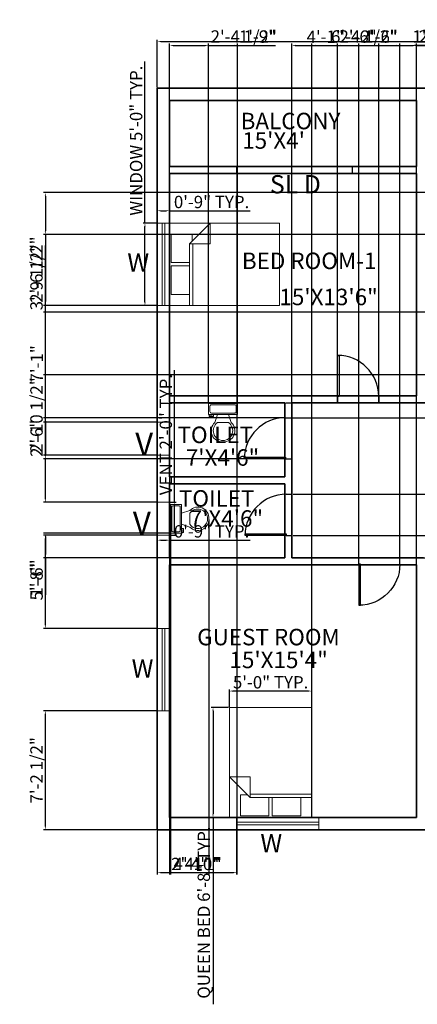
# Model space of a CAD drawing. Units: inches. Extents: x 3542 to 4275, y 1005 to 1722.
# Tile 1 of 6: x 3542 to 3831, y 1005 to 1722. Entities that reach past the tile are written whole.
import ezdxf

# ---------------------------------------------------------------- set-up
doc = ezdxf.new("R2010")
doc.units = ezdxf.units.IN
doc.layers.get('0').update_dxf_attribs({"color": 211})
for name, color, linetype, lineweight in [('A-ANNO-DIMS', 2, 'Continuous', 18), ('A-ANNO-TEXT', 7, 'Continuous', 18), ('A-AREA-IDEN', 7, 'Continuous', 25), ('A-DOOR', 3, 'Continuous', 25), ('A-FLOR-FIXT', 9, 'Continuous', 18), ('A-FURN', 8, 'Continuous', 18), ('A-GLAZ', 4, 'Continuous', 18), ('wall', 7, 'Continuous', 35)]:
    doc.layers.add(name, color=color, linetype=linetype, lineweight=lineweight)
doc.styles.get("Standard").update_dxf_attribs({"font": 'arial.ttf'})
doc.dimstyles.new('ISO-25', dxfattribs={"dimtxt": 9, "dimasz": 2.5, "dimexe": 1.25, "dimexo": 0.625, "dimtad": 1, "dimdec": 1, "dimlunit": 4, "dimtxsty": 'Standard', "dimcen": 2.5, "dimadec": 0, "dimazin": 0, "dimtfac": 1, "dimtdec": 1, "dimtmove": 0, "dimatfit": 3, "dimfxl": 1, "dimarcsym": 0})

# ---------------------------------------------------------------- blocks, each defined once
blk = doc.blocks.new('*U2')
for p, q in [((0, 0), (0, -6)), ((40, 0), (40, -6))]:
    blk.add_line(p, q)
blk.add_lwpolyline([(0, 0), (0, 40), (1.75, 40), (1.75, 0)], close=True)
blk.add_arc((0, 0), 40, 0, 90)
blk = doc.blocks.new('Bed - Queen')
for p, q in [((0, -80.00003), (0, 0)), ((0, 0), (59.99999, 0)), ((59.99999, 0), (59.99999, -80.00003)), ((7.99999, -1.2), (28.79998, -1.2)), ((7.99999, -14.4), (7.99999, -1.2)), ((28.79998, -1.2), (28.79998, -14.4)), ((31.19999, -1.2), (51.99999, -1.2)), ((31.19999, -14.4), (31.19999, -1.2)), ((51.99999, -1.2), (51.99999, -16.4)), ((0, -14.4), (44.8, -14.4)), ((44.8, -16.8), (0, -16.8)), ((59.99999, -29.6), (44.8, -14.4)), ((44.8, -14.4), (44.8, -29.6)), ((51.99999, -16.4), (46.79936, -16.4)), ((44.8, -29.6), (59.99999, -29.6)), ((59.99999, -80.00003), (0, -80.00003))]:
    blk.add_line(p, q)
blk = doc.blocks.new('*U11')
for p, q in [((9.5, -6), (9.5, -2)), ((-10, -8.5), (-8, -8.5)), ((-10, -9.5), (-10, -8.5)), ((-7, -9.5), (-10, -9.5)), ((-8, -8.5), (-8, -8)), ((-7, -8), (-7, -9.5)), ((-4, -8), (-6, -14)), ((4, -14), (-4, -14)), ((4, -8), (6, -14))]:
    blk.add_line(p, q)
blk.add_lwpolyline([(10.5, -8), (10.5, 0), (-10.5, 0), (-10.5, -8)], close=True)
for points in [[(-9.5, -2), (-9.5, -6)], [(8.5, -1), (-8.5, -1)], [(-8.5, -7), (8.5, -7)]]:
    blk.add_lwpolyline(points)
for centre, radius, start, end in [((-8.625, -1.875), 0.8839, 81.8699, 188.1301), ((-8.625, -6.125), 0.8839, 171.869898, 278.1301), ((8.625, -1.875), 0.8839, 351.8699, 98.1301), ((8.625, -6.125), 0.8839, 261.8699, 8.1301), ((-0.4772, -19.9188), 8.0953, 133.01722, 273.38), ((0.0374, -19.8731), 7.127, 124.50543, 269.7), ((-0.0373, -19.8731), 7.127, 270.3, 55.4946), ((0.4773, -19.9188), 8.0953, 266.62, 46.9828)]:
    blk.add_arc(centre, radius, start, end)
blk = doc.blocks.new('*D12')
at = {"layer": 'A-ANNO-DIMS', "color": 0, "lineweight": -2, "transparency": 16777216}
for p, q in [((3641.89, 1673.05), (3641.89, 1707.82)), ((4181.89, 1673.05), (4181.89, 1707.82)), ((3644.39, 1706.57), (4179.39, 1706.57))]:
    blk.add_line(p, q, dxfattribs=at)
at = {"layer": 'A-ANNO-DIMS', "color": 0, "transparency": 16777216}
for points in [[(3644.39, 1706.99), (3644.39, 1706.16), (3641.89, 1706.57)], [(4179.39, 1706.99), (4179.39, 1706.16), (4181.89, 1706.57)]]:
    blk.add_solid(points, dxfattribs=at)
at = {"layer": 'Defpoints', "color": 0, "transparency": 16777216}
for p in [(4181.89, 1706.57), (3641.89, 1672.43), (4181.89, 1672.43)]:
    blk.add_point(p, dxfattribs=at)
at = {"layer": 'A-ANNO-DIMS', "color": 0, "transparency": 16777216, "insert": (3911.89, 1711.77), "char_height": 9, "attachment_point": 5}
blk.add_mtext("45'", dxfattribs=at)
blk = doc.blocks.new('WIN-60IN')
for p, q in [((3.5, 60), (3.5, 0)), ((5.5, 60), (5.5, 0))]:
    blk.add_line(p, q)
blk.add_lwpolyline([(0, 60), (9, 60), (9, 0), (0, 0)], close=True)
blk = doc.blocks.new('DOOR-SLIDING-84IN')
blk.add_lwpolyline([(0, 0), (0, 5), (84, 5), (84, 0)], close=True)
blk = doc.blocks.new('VENT-24IN')
blk.add_lwpolyline([(0, 24), (9, 24), (9, 0), (0, 0)], close=True)
blk = doc.blocks.new('*D17')
at = {"layer": 'A-ANNO-DIMS', "color": 0, "lineweight": -2, "transparency": 16777216}
for p, q in [((3632.89, 1574.23), (3632.89, 1691.87)), ((3641.26, 1574.23), (3631.64, 1574.23)), ((3632.89, 1516.73), (3632.89, 1571.73)), ((3641.26, 1514.23), (3631.64, 1514.23))]:
    blk.add_line(p, q, dxfattribs=at)
at = {"layer": 'A-ANNO-DIMS', "color": 0, "transparency": 16777216}
for points in [[(3632.47, 1571.73), (3633.31, 1571.73), (3632.89, 1574.23)], [(3632.47, 1516.73), (3633.31, 1516.73), (3632.89, 1514.23)]]:
    blk.add_solid(points, dxfattribs=at)
at = {"layer": 'Defpoints', "color": 0, "transparency": 16777216}
for p in [(3632.89, 1574.23), (3641.89, 1574.23), (3641.89, 1514.23)]:
    blk.add_point(p, dxfattribs=at)
at = {"layer": 'A-ANNO-DIMS', "color": 0, "transparency": 16777216, "insert": (3627.61, 1634.3), "char_height": 9, "attachment_point": 5, "rotation": 90}
blk.add_mtext('WINDOW 5\'-0" TYP.', dxfattribs=at)
blk = doc.blocks.new('*D18')
at = {"layer": 'A-ANNO-DIMS', "color": 0, "lineweight": -2, "transparency": 16777216}
for p, q in [((3641.89, 1574.86), (3641.89, 1584.48)), ((3644.39, 1583.23), (3648.39, 1583.23)), ((3650.89, 1574.86), (3650.89, 1584.48)), ((3650.89, 1583.23), (3709.5, 1583.23))]:
    blk.add_line(p, q, dxfattribs=at)
at = {"layer": 'A-ANNO-DIMS', "color": 0, "transparency": 16777216}
for points in [[(3644.39, 1583.65), (3644.39, 1582.82), (3641.89, 1583.23)], [(3648.39, 1583.65), (3648.39, 1582.82), (3650.89, 1583.23)]]:
    blk.add_solid(points, dxfattribs=at)
at = {"layer": 'Defpoints', "color": 0, "transparency": 16777216}
for p in [(3650.89, 1583.23), (3641.89, 1574.23), (3650.89, 1574.23)]:
    blk.add_point(p, dxfattribs=at)
at = {"layer": 'A-ANNO-DIMS', "color": 0, "transparency": 16777216, "insert": (3681.44, 1588.45), "char_height": 9, "attachment_point": 5}
blk.add_mtext('0\'-9" TYP.', dxfattribs=at)
blk = doc.blocks.new('*D19')
at = {"layer": 'A-ANNO-DIMS', "color": 0, "lineweight": -2, "transparency": 16777216}
for p, q in [((3693.87, 1221.43), (3681.24, 1221.43)), ((3682.49, 1218.93), (3682.49, 1143.93)), ((3693.87, 1141.43), (3681.24, 1141.43)), ((3682.49, 1141.43), (3682.49, 1005.29))]:
    blk.add_line(p, q, dxfattribs=at)
at = {"layer": 'A-ANNO-DIMS', "color": 0, "transparency": 16777216}
for points in [[(3682.08, 1218.93), (3682.91, 1218.93), (3682.49, 1221.43)], [(3682.08, 1143.93), (3682.91, 1143.93), (3682.49, 1141.43)]]:
    blk.add_solid(points, dxfattribs=at)
at = {"layer": 'Defpoints', "color": 0, "transparency": 16777216}
for p in [(3694.49, 1221.43), (3682.49, 1141.43), (3694.49, 1141.43)]:
    blk.add_point(p, dxfattribs=at)
at = {"layer": 'A-ANNO-DIMS', "color": 0, "transparency": 16777216, "insert": (3676.94, 1072.11), "char_height": 9, "attachment_point": 5, "rotation": 90}
blk.add_mtext('QUEEN BED 6\'-8" TYP.', dxfattribs=at)
blk = doc.blocks.new('*D20')
at = {"layer": 'A-ANNO-DIMS', "color": 0, "lineweight": -2, "transparency": 16777216}
for p, q in [((3694.49, 1222.05), (3694.49, 1234.68)), ((3751.99, 1233.43), (3696.99, 1233.43)), ((3754.49, 1222.05), (3754.49, 1234.68))]:
    blk.add_line(p, q, dxfattribs=at)
at = {"layer": 'A-ANNO-DIMS', "color": 0, "transparency": 16777216}
for points in [[(3696.99, 1233.84), (3696.99, 1233.01), (3694.49, 1233.43)], [(3751.99, 1233.84), (3751.99, 1233.01), (3754.49, 1233.43)]]:
    blk.add_solid(points, dxfattribs=at)
at = {"layer": 'Defpoints', "color": 0, "transparency": 16777216}
for p in [(3694.49, 1233.43), (3694.49, 1221.43), (3754.49, 1221.43)]:
    blk.add_point(p, dxfattribs=at)
at = {"layer": 'A-ANNO-DIMS', "color": 0, "transparency": 16777216, "insert": (3724.49, 1238.65), "char_height": 9, "attachment_point": 5}
blk.add_mtext('5\'-0" TYP.', dxfattribs=at)
blk = doc.blocks.new('*D25')
at = {"layer": 'A-ANNO-DIMS', "color": 0, "lineweight": -2, "transparency": 16777216}
for p, q in [((3654.49, 1370.93), (3654.49, 1467.04)), ((3651.51, 1370.93), (3655.74, 1370.93)), ((3654.49, 1349.43), (3654.49, 1368.43)), ((3651.51, 1346.93), (3655.74, 1346.93))]:
    blk.add_line(p, q, dxfattribs=at)
at = {"layer": 'A-ANNO-DIMS', "color": 0, "transparency": 16777216}
for points in [[(3654.07, 1368.43), (3654.91, 1368.43), (3654.49, 1370.93)], [(3654.07, 1349.43), (3654.91, 1349.43), (3654.49, 1346.93)]]:
    blk.add_solid(points, dxfattribs=at)
at = {"layer": 'Defpoints', "color": 0, "transparency": 16777216}
for p in [(3650.89, 1370.93), (3654.49, 1370.93), (3650.89, 1346.93)]:
    blk.add_point(p, dxfattribs=at)
at = {"layer": 'A-ANNO-DIMS', "color": 0, "transparency": 16777216, "insert": (3649.27, 1420.23), "char_height": 9, "attachment_point": 5, "rotation": 90}
blk.add_mtext('VENT 2\'-0" TYP.', dxfattribs=at)
blk = doc.blocks.new('*D26')
at = {"layer": 'A-ANNO-DIMS', "color": 0, "lineweight": -2, "transparency": 16777216}
for p, q in [((3641.89, 1346.31), (3641.89, 1342.08)), ((3644.39, 1343.33), (3648.39, 1343.33)), ((3650.89, 1346.31), (3650.89, 1342.08)), ((3650.89, 1343.33), (3709.5, 1343.33))]:
    blk.add_line(p, q, dxfattribs=at)
at = {"layer": 'A-ANNO-DIMS', "color": 0, "transparency": 16777216}
for points in [[(3644.39, 1343.75), (3644.39, 1342.92), (3641.89, 1343.33)], [(3648.39, 1343.75), (3648.39, 1342.92), (3650.89, 1343.33)]]:
    blk.add_solid(points, dxfattribs=at)
at = {"layer": 'Defpoints', "color": 0, "transparency": 16777216}
for p in [(3641.89, 1346.93), (3650.89, 1346.93), (3650.89, 1343.33)]:
    blk.add_point(p, dxfattribs=at)
at = {"layer": 'A-ANNO-DIMS', "color": 0, "transparency": 16777216, "insert": (3681.44, 1348.55), "char_height": 9, "attachment_point": 5}
blk.add_mtext('0\'-9" TYP.', dxfattribs=at)
blk = doc.blocks.new('*D33')
at = {"layer": 'A-ANNO-DIMS', "color": 0, "lineweight": -2, "transparency": 16777216}
for p, q in [((3641.26, 1219.07), (3559.02, 1219.07)), ((3560.27, 1134.93), (3560.27, 1216.57)), ((3641.26, 1132.43), (3559.02, 1132.43))]:
    blk.add_line(p, q, dxfattribs=at)
at = {"layer": 'A-ANNO-DIMS', "color": 0, "transparency": 16777216}
for points in [[(3559.85, 1216.57), (3560.69, 1216.57), (3560.27, 1219.07)], [(3559.85, 1134.93), (3560.69, 1134.93), (3560.27, 1132.43)]]:
    blk.add_solid(points, dxfattribs=at)
at = {"layer": 'Defpoints', "color": 0, "transparency": 16777216}
for p in [(3560.27, 1219.07), (3641.89, 1219.07), (3641.89, 1132.43)]:
    blk.add_point(p, dxfattribs=at)
at = {"layer": 'A-ANNO-DIMS', "color": 0, "transparency": 16777216, "insert": (3554.99, 1175.75), "char_height": 9, "attachment_point": 5, "rotation": 90}
blk.add_mtext('7\'-2 1/2"', dxfattribs=at)
blk = doc.blocks.new('*D34')
at = {"layer": 'A-ANNO-DIMS', "color": 0, "lineweight": -2, "transparency": 16777216}
for p, q in [((3641.26, 1346.93), (3559.02, 1346.93)), ((3560.27, 1281.57), (3560.27, 1344.43)), ((3641.26, 1279.07), (3559.02, 1279.07))]:
    blk.add_line(p, q, dxfattribs=at)
at = {"layer": 'A-ANNO-DIMS', "color": 0, "transparency": 16777216}
for points in [[(3559.85, 1344.43), (3560.69, 1344.43), (3560.27, 1346.93)], [(3559.85, 1281.57), (3560.69, 1281.57), (3560.27, 1279.07)]]:
    blk.add_solid(points, dxfattribs=at)
at = {"layer": 'Defpoints', "color": 0, "transparency": 16777216}
for p in [(3560.27, 1346.93), (3641.89, 1346.93), (3641.89, 1279.07)]:
    blk.add_point(p, dxfattribs=at)
at = {"layer": 'A-ANNO-DIMS', "color": 0, "transparency": 16777216, "insert": (3555.05, 1313), "char_height": 9, "attachment_point": 5, "rotation": 90}
blk.add_mtext('5\'-8"', dxfattribs=at)
blk = doc.blocks.new('*D35')
at = {"layer": 'A-ANNO-DIMS', "color": 0, "lineweight": -2, "transparency": 16777216}
for p, q in [((3560.27, 1405.26), (3560.27, 1461.05)), ((3641.26, 1405.26), (3559.02, 1405.26)), ((3560.27, 1373.43), (3560.27, 1402.76)), ((3641.26, 1370.93), (3559.02, 1370.93))]:
    blk.add_line(p, q, dxfattribs=at)
at = {"layer": 'A-ANNO-DIMS', "color": 0, "transparency": 16777216}
for points in [[(3559.85, 1402.76), (3560.69, 1402.76), (3560.27, 1405.26)], [(3559.85, 1373.43), (3560.69, 1373.43), (3560.27, 1370.93)]]:
    blk.add_solid(points, dxfattribs=at)
at = {"layer": 'Defpoints', "color": 0, "transparency": 16777216}
for p in [(3560.27, 1405.26), (3641.89, 1405.26), (3641.89, 1370.93)]:
    blk.add_point(p, dxfattribs=at)
at = {"layer": 'A-ANNO-DIMS', "color": 0, "transparency": 16777216, "insert": (3554.99, 1434.41), "char_height": 9, "attachment_point": 5, "rotation": 90}
blk.add_mtext('2\'-10 1/2"', dxfattribs=at)
blk = doc.blocks.new('*D36')
at = {"layer": 'A-ANNO-DIMS', "color": 0, "lineweight": -2, "transparency": 16777216}
for p, q in [((3641.26, 1514.23), (3559.02, 1514.23)), ((3560.27, 1431.76), (3560.27, 1511.73)), ((3641.26, 1429.26), (3559.02, 1429.26))]:
    blk.add_line(p, q, dxfattribs=at)
at = {"layer": 'A-ANNO-DIMS', "color": 0, "transparency": 16777216}
for points in [[(3559.85, 1511.73), (3560.69, 1511.73), (3560.27, 1514.23)], [(3559.85, 1431.76), (3560.69, 1431.76), (3560.27, 1429.26)]]:
    blk.add_solid(points, dxfattribs=at)
at = {"layer": 'Defpoints', "color": 0, "transparency": 16777216}
for p in [(3560.27, 1514.23), (3641.89, 1514.23), (3641.89, 1429.26)]:
    blk.add_point(p, dxfattribs=at)
at = {"layer": 'A-ANNO-DIMS', "color": 0, "transparency": 16777216, "insert": (3555.13, 1471.75), "char_height": 9, "attachment_point": 5, "rotation": 90}
blk.add_mtext('7\'-1"', dxfattribs=at)
blk = doc.blocks.new('*D37')
at = {"layer": 'A-ANNO-DIMS', "color": 0, "lineweight": -2, "transparency": 16777216}
for p, q in [((3641.89, 1131.8), (3641.89, 1099.93)), ((3699.65, 1131.8), (3699.65, 1099.93)), ((3644.39, 1101.18), (3697.15, 1101.18))]:
    blk.add_line(p, q, dxfattribs=at)
at = {"layer": 'A-ANNO-DIMS', "color": 0, "transparency": 16777216}
for points in [[(3644.39, 1101.59), (3644.39, 1100.76), (3641.89, 1101.18)], [(3697.15, 1101.59), (3697.15, 1100.76), (3699.65, 1101.18)]]:
    blk.add_solid(points, dxfattribs=at)
at = {"layer": 'Defpoints', "color": 0, "transparency": 16777216}
for p in [(3641.89, 1132.43), (3699.65, 1132.43), (3699.65, 1101.18)]:
    blk.add_point(p, dxfattribs=at)
at = {"layer": 'A-ANNO-DIMS', "color": 0, "transparency": 16777216, "insert": (3670.77, 1106.4), "char_height": 9, "attachment_point": 5}
blk.add_mtext('4\'-10"', dxfattribs=at)
blk = doc.blocks.new('*D42')
at = {"layer": 'A-ANNO-DIMS', "color": 0, "lineweight": -2, "transparency": 16777216}
for p, q in [((3650.89, 1609.8), (3650.89, 1099.93)), ((3699.86, 1609.8), (3699.86, 1099.93)), ((3653.39, 1101.18), (3697.36, 1101.18))]:
    blk.add_line(p, q, dxfattribs=at)
at = {"layer": 'A-ANNO-DIMS', "color": 0, "transparency": 16777216}
for points in [[(3653.39, 1101.59), (3653.39, 1100.76), (3650.89, 1101.18)], [(3697.36, 1101.59), (3697.36, 1100.76), (3699.86, 1101.18)]]:
    blk.add_solid(points, dxfattribs=at)
at = {"layer": 'Defpoints', "color": 0, "transparency": 16777216}
for p in [(3650.89, 1610.43), (3699.86, 1610.43), (3699.86, 1101.18)]:
    blk.add_point(p, dxfattribs=at)
at = {"layer": 'A-ANNO-DIMS', "color": 0, "transparency": 16777216, "insert": (3675.37, 1106.32), "char_height": 9, "attachment_point": 5}
blk.add_mtext('4\'-1"', dxfattribs=at)
blk = doc.blocks.new('*D45')
at = {"layer": 'A-ANNO-DIMS', "color": 0, "lineweight": -2, "transparency": 16777216}
for p, q in [((3773.24, 1444.05), (3773.24, 1704.93)), ((3775.74, 1703.68), (3800.74, 1703.68)), ((3803.24, 1444.05), (3803.24, 1704.93))]:
    blk.add_line(p, q, dxfattribs=at)
at = {"layer": 'A-ANNO-DIMS', "color": 0, "transparency": 16777216}
for points in [[(3775.74, 1704.09), (3775.74, 1703.26), (3773.24, 1703.68)], [(3800.74, 1704.09), (3800.74, 1703.26), (3803.24, 1703.68)]]:
    blk.add_solid(points, dxfattribs=at)
at = {"layer": 'Defpoints', "color": 0, "transparency": 16777216}
for p in [(3803.24, 1703.68), (3773.24, 1443.43), (3803.24, 1443.43)]:
    blk.add_point(p, dxfattribs=at)
at = {"layer": 'A-ANNO-DIMS', "color": 0, "transparency": 16777216, "insert": (3788.24, 1708.9), "char_height": 9, "attachment_point": 5}
blk.add_mtext('2\'-6"', dxfattribs=at)
blk = doc.blocks.new('*D46')
at = {"layer": 'A-ANNO-DIMS', "color": 0, "lineweight": -2, "transparency": 16777216}
for p, q in [((3803.24, 1444.05), (3803.24, 1704.93)), ((3805.74, 1703.68), (3828.39, 1703.68)), ((3830.89, 1449.05), (3830.89, 1704.93)), ((3830.89, 1703.68), (3879.69, 1703.68))]:
    blk.add_line(p, q, dxfattribs=at)
at = {"layer": 'A-ANNO-DIMS', "color": 0, "transparency": 16777216}
for points in [[(3805.74, 1704.09), (3805.74, 1703.26), (3803.24, 1703.68)], [(3828.39, 1704.09), (3828.39, 1703.26), (3830.89, 1703.68)]]:
    blk.add_solid(points, dxfattribs=at)
at = {"layer": 'Defpoints', "color": 0, "transparency": 16777216}
for p in [(3830.89, 1703.68), (3803.24, 1443.43), (3830.89, 1448.43)]:
    blk.add_point(p, dxfattribs=at)
at = {"layer": 'A-ANNO-DIMS', "color": 0, "transparency": 16777216, "insert": (3856.54, 1708.96), "char_height": 9, "attachment_point": 5}
blk.add_mtext('2\'-3 1/2"', dxfattribs=at)
blk = doc.blocks.new('*D54')
at = {"layer": 'A-ANNO-DIMS', "color": 0, "lineweight": -2, "transparency": 16777216}
for p, q in [((4047.2, 1596.46), (3559.02, 1596.46)), ((3560.27, 1593.96), (3560.27, 1568.52)), ((4047.2, 1566.02), (3559.02, 1566.02)), ((3560.27, 1566.02), (3560.27, 1517.22))]:
    blk.add_line(p, q, dxfattribs=at)
at = {"layer": 'A-ANNO-DIMS', "color": 0, "transparency": 16777216}
for points in [[(3559.85, 1593.96), (3560.69, 1593.96), (3560.27, 1596.46)], [(3559.85, 1568.52), (3560.69, 1568.52), (3560.27, 1566.02)]]:
    blk.add_solid(points, dxfattribs=at)
at = {"layer": 'Defpoints', "color": 0, "transparency": 16777216}
for p in [(4047.82, 1596.46), (3560.27, 1566.02), (4047.82, 1566.02)]:
    blk.add_point(p, dxfattribs=at)
at = {"layer": 'A-ANNO-DIMS', "color": 0, "transparency": 16777216, "insert": (3554.99, 1540.37), "char_height": 9, "attachment_point": 5, "rotation": 90}
blk.add_mtext('2\'-6 1/2"', dxfattribs=at)
blk = doc.blocks.new('*D55')
at = {"layer": 'A-ANNO-DIMS', "color": 0, "lineweight": -2, "transparency": 16777216}
for p, q in [((3560.27, 1509.3), (3560.27, 1557.94)), ((4047.2, 1509.3), (3559.02, 1509.3)), ((3560.27, 1466.15), (3560.27, 1506.8)), ((4047.2, 1463.65), (3559.02, 1463.65))]:
    blk.add_line(p, q, dxfattribs=at)
at = {"layer": 'A-ANNO-DIMS', "color": 0, "transparency": 16777216}
for points in [[(3559.85, 1506.8), (3560.69, 1506.8), (3560.27, 1509.3)], [(3559.85, 1466.15), (3560.69, 1466.15), (3560.27, 1463.65)]]:
    blk.add_solid(points, dxfattribs=at)
at = {"layer": 'Defpoints', "color": 0, "transparency": 16777216}
for p in [(3560.27, 1509.3), (4047.82, 1509.3), (4047.82, 1463.65)]:
    blk.add_point(p, dxfattribs=at)
at = {"layer": 'A-ANNO-DIMS', "color": 0, "transparency": 16777216, "insert": (3554.99, 1534.87), "char_height": 9, "attachment_point": 5, "rotation": 90}
blk.add_mtext('3\'-9 1/2"', dxfattribs=at)
blk = doc.blocks.new('*D61')
at = {"layer": 'A-ANNO-DIMS', "color": 0, "lineweight": -2, "transparency": 16777216}
for p, q in [((3877.16, 1703.68), (3829.36, 1703.68)), ((3877.16, 1207.47), (3877.16, 1704.93)), ((3893.39, 1703.68), (3879.66, 1703.68)), ((3895.89, 1207.05), (3895.89, 1704.93))]:
    blk.add_line(p, q, dxfattribs=at)
at = {"layer": 'A-ANNO-DIMS', "color": 0, "transparency": 16777216}
for points in [[(3879.66, 1704.09), (3879.66, 1703.26), (3877.16, 1703.68)], [(3893.39, 1704.09), (3893.39, 1703.26), (3895.89, 1703.68)]]:
    blk.add_solid(points, dxfattribs=at)
at = {"layer": 'Defpoints', "color": 0, "transparency": 16777216}
for p in [(3877.16, 1703.68), (3877.16, 1206.85), (3895.89, 1206.43)]:
    blk.add_point(p, dxfattribs=at)
at = {"layer": 'A-ANNO-DIMS', "color": 0, "transparency": 16777216, "insert": (3852.01, 1708.96), "char_height": 9, "attachment_point": 5}
blk.add_mtext('1\'-6 1/2"', dxfattribs=at)
blk = doc.blocks.new('*D62')
at = {"layer": 'A-ANNO-DIMS', "color": 0, "lineweight": -2, "transparency": 16777216}
for p, q in [((3739.89, 1331.05), (3739.89, 1704.93)), ((3742.39, 1703.68), (3786.19, 1703.68)), ((3788.69, 1330.99), (3788.69, 1704.93))]:
    blk.add_line(p, q, dxfattribs=at)
at = {"layer": 'A-ANNO-DIMS', "color": 0, "transparency": 16777216}
for points in [[(3742.39, 1704.09), (3742.39, 1703.26), (3739.89, 1703.68)], [(3786.19, 1704.09), (3786.19, 1703.26), (3788.69, 1703.68)]]:
    blk.add_solid(points, dxfattribs=at)
at = {"layer": 'Defpoints', "color": 0, "transparency": 16777216}
for p in [(3788.69, 1703.68), (3739.89, 1330.43), (3788.69, 1330.37)]:
    blk.add_point(p, dxfattribs=at)
at = {"layer": 'A-ANNO-DIMS', "color": 0, "transparency": 16777216, "insert": (3764.29, 1708.82), "char_height": 9, "attachment_point": 5}
blk.add_mtext('4\'-1"', dxfattribs=at)
blk = doc.blocks.new('*D63')
at = {"layer": 'A-ANNO-DIMS', "color": 0, "lineweight": -2, "transparency": 16777216}
for p, q in [((3788.69, 1330.99), (3788.69, 1704.93)), ((3791.19, 1703.68), (3816.19, 1703.68)), ((3818.69, 1330.99), (3818.69, 1704.93))]:
    blk.add_line(p, q, dxfattribs=at)
at = {"layer": 'A-ANNO-DIMS', "color": 0, "transparency": 16777216}
for points in [[(3791.19, 1704.09), (3791.19, 1703.26), (3788.69, 1703.68)], [(3816.19, 1704.09), (3816.19, 1703.26), (3818.69, 1703.68)]]:
    blk.add_solid(points, dxfattribs=at)
at = {"layer": 'Defpoints', "color": 0, "transparency": 16777216}
for p in [(3818.69, 1703.68), (3788.69, 1330.37), (3818.69, 1330.37)]:
    blk.add_point(p, dxfattribs=at)
at = {"layer": 'A-ANNO-DIMS', "color": 0, "transparency": 16777216, "insert": (3803.69, 1708.9), "char_height": 9, "attachment_point": 5}
blk.add_mtext('2\'-6"', dxfattribs=at)
blk = doc.blocks.new('*D64')
at = {"layer": 'A-ANNO-DIMS', "color": 0, "lineweight": -2, "transparency": 16777216}
for p, q in [((3741.01, 1376.72), (4214.39, 1376.72)), ((4213.14, 1374.22), (4213.14, 1349.22)), ((3741.01, 1346.72), (4214.39, 1346.72))]:
    blk.add_line(p, q, dxfattribs=at)
at = {"layer": 'A-ANNO-DIMS', "color": 0, "transparency": 16777216}
for points in [[(4212.72, 1374.22), (4213.56, 1374.22), (4213.14, 1376.72)], [(4212.72, 1349.22), (4213.56, 1349.22), (4213.14, 1346.72)]]:
    blk.add_solid(points, dxfattribs=at)
at = {"layer": 'Defpoints', "color": 0, "transparency": 16777216}
for p in [(3740.38, 1376.72), (3740.38, 1346.72), (4213.14, 1346.72)]:
    blk.add_point(p, dxfattribs=at)
at = {"layer": 'A-ANNO-DIMS', "color": 0, "transparency": 16777216, "insert": (4207.92, 1361.72), "char_height": 9, "attachment_point": 5, "rotation": 90}
blk.add_mtext('2\'-6"', dxfattribs=at)
blk = doc.blocks.new('*D65')
at = {"layer": 'A-ANNO-DIMS', "color": 0, "lineweight": -2, "transparency": 16777216}
for p, q in [((3734.7, 1432.53), (3559.02, 1432.53)), ((3560.27, 1430.03), (3560.27, 1405.03)), ((3734.7, 1402.53), (3559.02, 1402.53))]:
    blk.add_line(p, q, dxfattribs=at)
at = {"layer": 'A-ANNO-DIMS', "color": 0, "transparency": 16777216}
for points in [[(3559.85, 1430.03), (3560.69, 1430.03), (3560.27, 1432.53)], [(3559.85, 1405.03), (3560.69, 1405.03), (3560.27, 1402.53)]]:
    blk.add_solid(points, dxfattribs=at)
at = {"layer": 'Defpoints', "color": 0, "transparency": 16777216}
for p in [(3735.32, 1432.53), (3560.27, 1402.53), (3735.32, 1402.53)]:
    blk.add_point(p, dxfattribs=at)
at = {"layer": 'A-ANNO-DIMS', "color": 0, "transparency": 16777216, "insert": (3555.05, 1417.53), "char_height": 9, "attachment_point": 5, "rotation": 90}
blk.add_mtext('2\'-6"', dxfattribs=at)
blk = doc.blocks.new('*D66')
at = {"layer": 'A-ANNO-DIMS', "color": 0, "lineweight": -2, "transparency": 16777216}
for p, q in [((3735.51, 1443.43), (4214.39, 1443.43)), ((4213.14, 1440.93), (4213.14, 1435.03)), ((3735.95, 1432.53), (4214.39, 1432.53)), ((4213.14, 1432.53), (4213.14, 1397.86))]:
    blk.add_line(p, q, dxfattribs=at)
at = {"layer": 'A-ANNO-DIMS', "color": 0, "transparency": 16777216}
for points in [[(4212.72, 1440.93), (4213.56, 1440.93), (4213.14, 1443.43)], [(4212.72, 1435.03), (4213.56, 1435.03), (4213.14, 1432.53)]]:
    blk.add_solid(points, dxfattribs=at)
at = {"layer": 'Defpoints', "color": 0, "transparency": 16777216}
for p in [(3734.89, 1443.43), (3735.32, 1432.53), (4213.14, 1432.53)]:
    blk.add_point(p, dxfattribs=at)
at = {"layer": 'A-ANNO-DIMS', "color": 0, "transparency": 16777216, "insert": (4207.92, 1413.94), "char_height": 9, "attachment_point": 5, "rotation": 90}
blk.add_mtext('0\'-11"', dxfattribs=at)
blk = doc.blocks.new('*D67')
at = {"layer": 'A-ANNO-DIMS', "color": 0, "lineweight": -2, "transparency": 16777216}
for p, q in [((4213.14, 1346.72), (4213.14, 1394.52)), ((3741.01, 1346.72), (4214.39, 1346.72)), ((4213.14, 1332.93), (4213.14, 1344.22)), ((3740.51, 1330.43), (4214.39, 1330.43))]:
    blk.add_line(p, q, dxfattribs=at)
at = {"layer": 'A-ANNO-DIMS', "color": 0, "transparency": 16777216}
for points in [[(4212.72, 1344.22), (4213.56, 1344.22), (4213.14, 1346.72)], [(4212.72, 1332.93), (4213.56, 1332.93), (4213.14, 1330.43)]]:
    blk.add_solid(points, dxfattribs=at)
at = {"layer": 'Defpoints', "color": 0, "transparency": 16777216}
for p in [(3740.38, 1346.72), (4213.14, 1346.72), (3739.89, 1330.43)]:
    blk.add_point(p, dxfattribs=at)
at = {"layer": 'A-ANNO-DIMS', "color": 0, "transparency": 16777216, "insert": (4207.86, 1371.87), "char_height": 9, "attachment_point": 5, "rotation": 90}
blk.add_mtext('1\'-4 1/2"', dxfattribs=at)
blk = doc.blocks.new('*D68')
at = {"layer": 'A-ANNO-DIMS', "color": 0, "lineweight": -2, "transparency": 16777216}
for p, q in [((3679.29, 1443.55), (3679.29, 1704.93)), ((3681.79, 1703.68), (3697.79, 1703.68)), ((3700.29, 1443.55), (3700.29, 1704.93)), ((3700.29, 1703.68), (3727.12, 1703.68))]:
    blk.add_line(p, q, dxfattribs=at)
at = {"layer": 'A-ANNO-DIMS', "color": 0, "transparency": 16777216}
for points in [[(3681.79, 1704.09), (3681.79, 1703.26), (3679.29, 1703.68)], [(3697.79, 1704.09), (3697.79, 1703.26), (3700.29, 1703.68)]]:
    blk.add_solid(points, dxfattribs=at)
at = {"layer": 'Defpoints', "color": 0, "transparency": 16777216}
for p in [(3700.29, 1703.68), (3679.29, 1442.92), (3700.29, 1442.92)]:
    blk.add_point(p, dxfattribs=at)
at = {"layer": 'A-ANNO-DIMS', "color": 0, "transparency": 16777216, "insert": (3714.96, 1708.9), "char_height": 9, "attachment_point": 5}
blk.add_mtext('1\'-9"', dxfattribs=at)
blk = doc.blocks.new('*D69')
at = {"layer": 'A-ANNO-DIMS', "color": 0, "lineweight": -2, "transparency": 16777216}
for p, q in [((3650.89, 1444.05), (3650.89, 1704.93)), ((3653.39, 1703.68), (3676.79, 1703.68)), ((3679.29, 1443.55), (3679.29, 1704.93)), ((3679.29, 1703.68), (3728.09, 1703.68))]:
    blk.add_line(p, q, dxfattribs=at)
at = {"layer": 'A-ANNO-DIMS', "color": 0, "transparency": 16777216}
for points in [[(3653.39, 1704.09), (3653.39, 1703.26), (3650.89, 1703.68)], [(3676.79, 1704.09), (3676.79, 1703.26), (3679.29, 1703.68)]]:
    blk.add_solid(points, dxfattribs=at)
at = {"layer": 'Defpoints', "color": 0, "transparency": 16777216}
for p in [(3679.29, 1703.68), (3650.89, 1443.43), (3679.29, 1442.92)]:
    blk.add_point(p, dxfattribs=at)
at = {"layer": 'A-ANNO-DIMS', "color": 0, "transparency": 16777216, "insert": (3704.94, 1708.96), "char_height": 9, "attachment_point": 5}
blk.add_mtext('2\'-4 1/2"', dxfattribs=at)
blk = doc.blocks.new('*D70')
at = {"layer": 'A-ANNO-DIMS', "color": 0, "lineweight": -2, "transparency": 16777216}
for p, q in [((3651.52, 1368.77), (3651.52, 1099.93)), ((3679.52, 1358.27), (3679.52, 1099.93)), ((3654.02, 1101.18), (3677.02, 1101.18))]:
    blk.add_line(p, q, dxfattribs=at)
at = {"layer": 'A-ANNO-DIMS', "color": 0, "transparency": 16777216}
for points in [[(3654.02, 1101.59), (3654.02, 1100.76), (3651.52, 1101.18)], [(3677.02, 1101.59), (3677.02, 1100.76), (3679.52, 1101.18)]]:
    blk.add_solid(points, dxfattribs=at)
at = {"layer": 'Defpoints', "color": 0, "transparency": 16777216}
for p in [(3651.52, 1369.4), (3679.52, 1358.9), (3679.52, 1101.18)]:
    blk.add_point(p, dxfattribs=at)
at = {"layer": 'A-ANNO-DIMS', "color": 0, "transparency": 16777216, "insert": (3665.52, 1106.32), "char_height": 9, "attachment_point": 5}
blk.add_mtext('2\'-4"', dxfattribs=at)
blk = doc.blocks.new('*D71')
at = {"layer": 'A-ANNO-DIMS', "color": 0, "lineweight": -2, "transparency": 16777216}
for p, q in [((3650.89, 1348.4), (3559.02, 1348.4)), ((3560.27, 1345.9), (3560.27, 1332.93)), ((3650.26, 1330.43), (3559.02, 1330.43)), ((3560.27, 1330.43), (3560.27, 1303.6))]:
    blk.add_line(p, q, dxfattribs=at)
at = {"layer": 'A-ANNO-DIMS', "color": 0, "transparency": 16777216}
for points in [[(3559.85, 1345.9), (3560.69, 1345.9), (3560.27, 1348.4)], [(3559.85, 1332.93), (3560.69, 1332.93), (3560.27, 1330.43)]]:
    blk.add_solid(points, dxfattribs=at)
at = {"layer": 'Defpoints', "color": 0, "transparency": 16777216}
for p in [(3651.52, 1348.4), (3560.27, 1330.43), (3650.89, 1330.43)]:
    blk.add_point(p, dxfattribs=at)
at = {"layer": 'A-ANNO-DIMS', "color": 0, "transparency": 16777216, "insert": (3555.05, 1315.76), "char_height": 9, "attachment_point": 5, "rotation": 90}
blk.add_mtext('1\'-6"', dxfattribs=at)
blk = doc.blocks.new('*D72')
at = {"layer": 'A-ANNO-DIMS', "color": 0, "lineweight": -2, "transparency": 16777216}
for p, q in [((3754.49, 1142.05), (3754.49, 1704.93)), ((3756.99, 1703.68), (3828.39, 1703.68)), ((3830.89, 1142.05), (3830.89, 1704.93))]:
    blk.add_line(p, q, dxfattribs=at)
at = {"layer": 'A-ANNO-DIMS', "color": 0, "transparency": 16777216}
for points in [[(3756.99, 1704.09), (3756.99, 1703.26), (3754.49, 1703.68)], [(3828.39, 1704.09), (3828.39, 1703.26), (3830.89, 1703.68)]]:
    blk.add_solid(points, dxfattribs=at)
at = {"layer": 'Defpoints', "color": 0, "transparency": 16777216}
for p in [(3830.89, 1703.68), (3754.49, 1141.43), (3830.89, 1141.43)]:
    blk.add_point(p, dxfattribs=at)
at = {"layer": 'A-ANNO-DIMS', "color": 0, "transparency": 16777216, "insert": (3792.69, 1708.96), "char_height": 9, "attachment_point": 5}
blk.add_mtext('6\'-4 1/2"', dxfattribs=at)

msp = doc.modelspace()

# ---------------------------------------------------------------- linework, layer by layer
at = {"layer": 'wall'}
for p, q in [((3641.89, 1672.43), (4181.89, 1672.43)), ((3641.89, 1132.43), (3641.89, 1672.43)), ((3650.89, 1663.43), (3830.89, 1663.43)), ((3650.89, 1615.43), (3650.89, 1663.43)), ((3830.89, 1615.43), (3830.89, 1663.43)), ((3650.89, 1615.43), (3830.89, 1615.43)), ((3650.89, 1610.43), (3830.89, 1610.43)), ((3650.89, 1448.43), (3650.89, 1610.43)), ((3830.89, 1448.43), (3830.89, 1610.43)), ((3650.89, 1448.43), (3830.89, 1448.43)), ((3650.89, 1443.43), (3734.89, 1443.43)), ((3650.89, 1389.43), (3650.89, 1443.43)), ((3734.89, 1389.43), (3734.89, 1443.43)), ((3739.89, 1443.43), (4058.5, 1443.43)), ((3739.89, 1384.43), (3739.89, 1443.43)), ((3739.89, 1443.43), (3830.89, 1443.43)), ((3650.89, 1389.43), (3734.89, 1389.43)), ((3650.89, 1384.43), (3734.89, 1384.43)), ((3650.89, 1330.43), (3650.89, 1384.43)), ((3734.89, 1330.43), (3734.89, 1384.43)), ((3739.89, 1330.43), (3739.89, 1384.43)), ((3650.89, 1330.43), (3734.89, 1330.43)), ((3739.89, 1330.43), (3835.89, 1330.43)), ((3650.89, 1141.43), (3650.89, 1325.43)), ((3650.89, 1325.43), (3830.89, 1325.43)), ((3830.89, 1141.43), (3830.89, 1325.43)), ((3830.89, 1141.43), (3650.89, 1141.43)), ((4181.89, 1132.43), (3641.89, 1132.43))]:
    msp.add_line(p, q, dxfattribs=at)

# ---------------------------------------------------------------- block references
at = {"layer": 'A-DOOR'}
msp.add_blockref('DOOR-SLIDING-84IN', (3699.86, 1610.43), dxfattribs=at)
at = {"layer": 'A-DOOR', "xscale": 0.75, "yscale": 0.75, "zscale": 0.75}
msp.add_blockref('*U2', (3773.24, 1447.93), dxfattribs=at)
at = {"layer": 'A-DOOR', "yscale": 0.75, "zscale": 0.75}
for p, xscale, rotation in [((3735.32, 1402.53), 0.75, 90), ((3735.88, 1346.72), 0.75, 90), ((3788.69, 1325.87), -0.75, 180)]:
    msp.add_blockref('*U2', p, dxfattribs=dict(at, xscale=xscale, rotation=rotation))
at = {"layer": 'A-FLOR-FIXT'}
msp.add_blockref('*U11', (3689.79, 1442.92), dxfattribs=at)
at = {"layer": 'A-FLOR-FIXT', "rotation": 90}
msp.add_blockref('*U11', (3651.52, 1358.9), dxfattribs=at)
at = {"layer": 'A-FURN'}
for p, rotation in [((3650.89, 1514.23), 90), ((3754.49, 1141.43), 180)]:
    msp.add_blockref('Bed - Queen', p, dxfattribs=dict(at, rotation=rotation))
at = {"layer": 'A-GLAZ'}
for name, p in [('WIN-60IN', (3641.89, 1514.23)), ('VENT-24IN', (3641.89, 1405.26)), ('VENT-24IN', (3641.89, 1346.93)), ('WIN-60IN', (3641.89, 1219.07))]:
    msp.add_blockref(name, p, dxfattribs=at)
at = {"layer": 'A-GLAZ', "rotation": 90.00000000000033}
msp.add_blockref('WIN-60IN', (3759.65, 1132.43), dxfattribs=at)

# ---------------------------------------------------------------- texts
at = {"layer": 'A-ANNO-TEXT'}
for s, height, p in [('SL D', 13.276, (3723.96, 1595.9)), ('W', 13.28, (3620.05, 1538.92)), ('V', 16.64, (3625.79, 1405.09)), ('V', 16.64, (3624.1, 1347.34)), ('W', 13.28, (3623.18, 1243.27)), ('W', 13.28, (3717.01, 1116.05))]:
    msp.add_text(s, height=height, dxfattribs=at).set_placement(p)
at = {"layer": 'A-AREA-IDEN'}
for s, p in [('BALCONY', (3702.62, 1642.59)), ("15'X4'", (3703.76, 1628.39)), ('BED ROOM-1', (3703.53, 1540.75)), ('15\'X13\'6"', (3730.89, 1514.45)), ('TOILET', (3656.6, 1414.02)), ('7\'X4\'6"', (3662.67, 1397.5)), ('TOILET', (3657.64, 1367.73)), ('7\'X4\'6"', (3665.52, 1353.1)), ('GUEST ROOM', (3670.94, 1266.74)), ('15\'X15\'4"', (3694.49, 1250.1))]:
    msp.add_text(s, height=12, dxfattribs=at).set_placement(p)

# ---------------------------------------------------------------- dimensions: what is measured, and where the dimension line sits
at = {"layer": 'A-ANNO-DIMS'}
for base, p1, p2, override, picture, middle in [((3679.29, 1703.68), (3650.89, 1443.43), (3679.29, 1442.92), {"dimdec": 1, "dimlfac": 1, "dimrnd": 0, "dimzin": 1, "dimdsep": 46, "dimlunit": 4, "dimfrac": 2}, '*D69', (3704.94, 1708.96)), ((3830.89, 1703.68), (3754.49, 1141.43), (3830.89, 1141.43), {"dimdec": 1, "dimlfac": 1, "dimrnd": 0, "dimzin": 1, "dimdsep": 46, "dimlunit": 4, "dimfrac": 2}, '*D72', (3792.69, 1708.96)), ((3830.8894, 1703.6779), (3803.2386, 1443.4279), (3830.8894, 1448.4279), {"dimdec": 1, "dimlfac": 1, "dimrnd": 0, "dimzin": 1, "dimdsep": 46, "dimlunit": 4, "dimfrac": 2}, '*D46', (3856.5389, 1708.9594)), ((3877.16, 1703.68), (3895.89, 1206.43), (3877.16, 1206.85), {"dimdec": 1, "dimlfac": 1, "dimrnd": 0, "dimzin": 1, "dimdsep": 46, "dimlunit": 4, "dimfrac": 2}, '*D61', (3852.01, 1708.96)), ((4181.89, 1706.57), (3641.89, 1672.43), (4181.89, 1672.43), {"dimclrd": 0, "dimclre": 0, "dimclrt": 0}, '*D12', (3911.89, 1711.77)), ((3700.29, 1703.68), (3679.29, 1442.92), (3700.29, 1442.92), {"dimdec": 1, "dimlfac": 1, "dimrnd": 0, "dimzin": 1, "dimdsep": 46, "dimlunit": 4, "dimfrac": 2}, '*D68', (3714.96, 1708.9)), ((3788.69, 1703.68), (3739.89, 1330.43), (3788.69, 1330.37), {"dimdec": 1, "dimlfac": 1, "dimrnd": 0, "dimzin": 1, "dimdsep": 46, "dimlunit": 4, "dimfrac": 2}, '*D62', (3764.29, 1708.82)), ((3803.24, 1703.68), (3773.24, 1443.43), (3803.24, 1443.43), {"dimdec": 1, "dimlfac": 1, "dimrnd": 0, "dimzin": 1, "dimdsep": 46, "dimlunit": 4, "dimfrac": 2}, '*D45', (3788.24, 1708.9)), ((3818.69, 1703.68), (3788.69, 1330.37), (3818.69, 1330.37), {"dimdec": 1, "dimlfac": 1, "dimrnd": 0, "dimzin": 1, "dimdsep": 46, "dimlunit": 4, "dimfrac": 2}, '*D63', (3803.69, 1708.9)), ((3699.86, 1101.18), (3650.89, 1610.43), (3699.86, 1610.43), {"dimdec": 1, "dimlfac": 1, "dimrnd": 0, "dimzin": 1, "dimdsep": 46, "dimlunit": 4, "dimfrac": 2}, '*D42', (3675.37, 1106.32)), ((3679.52, 1101.18), (3651.52, 1369.4), (3679.52, 1358.9), {"dimdec": 1, "dimlfac": 1, "dimrnd": 0, "dimzin": 1, "dimdsep": 46, "dimlunit": 4, "dimfrac": 2}, '*D70', (3665.52, 1106.32)), ((3699.65, 1101.18), (3641.89, 1132.43), (3699.65, 1132.43), {"dimdec": 1, "dimlfac": 1, "dimrnd": 0, "dimzin": 1, "dimdsep": 46, "dimlunit": 4, "dimfrac": 2}, '*D37', (3670.77, 1106.4))]:
    dim = msp.add_linear_dim(base=base, p1=p1, p2=p2, dimstyle='ISO-25', override=override, dxfattribs=at)
    dim.commit()
    dim.dimension.update_dxf_attribs({"geometry": picture, "text_midpoint": middle})
for base, p1, p2, angle, text, picture, middle in [((3632.89, 1574.23), (3641.89, 1514.23), (3641.89, 1574.23), 90, 'WINDOW <> TYP.', '*D17', (3627.61, 1634.3)), ((3654.49, 1370.93), (3650.89, 1346.93), (3650.89, 1370.93), 90, 'VENT <> TYP.', '*D25', (3649.27, 1420.23)), ((3694.49, 1233.43), (3754.49, 1221.43), (3694.49, 1221.43), 180, '<> TYP.', '*D20', (3724.49, 1238.65)), ((3682.49, 1141.43), (3694.49, 1221.43), (3694.49, 1141.43), 270, 'QUEEN BED <> TYP.', '*D19', (3676.94, 1072.11))]:
    dim = msp.add_linear_dim(base=base, p1=p1, p2=p2, angle=angle, text=text, dimstyle='ISO-25', override={"dimdec": 1, "dimlfac": 1, "dimrnd": 0, "dimzin": 1, "dimdsep": 46, "dimlunit": 4, "dimfrac": 2}, dxfattribs=at)
    dim.commit()
    dim.dimension.update_dxf_attribs({"geometry": picture, "text_midpoint": middle})
for base, p1, p2, picture, middle in [((3650.89, 1583.23), (3641.89, 1574.23), (3650.89, 1574.23), '*D18', (3681.44, 1588.45)), ((3650.89, 1343.33), (3641.89, 1346.93), (3650.89, 1346.93), '*D26', (3681.44, 1348.55))]:
    dim = msp.add_linear_dim(base=base, p1=p1, p2=p2, text='<> TYP.', dimstyle='ISO-25', override={"dimdec": 1, "dimlfac": 1, "dimrnd": 0, "dimzin": 1, "dimdsep": 46, "dimlunit": 4, "dimfrac": 2}, dxfattribs=at)
    dim.commit()
    dim.dimension.update_dxf_attribs({"geometry": picture, "text_midpoint": middle})
for base, p1, p2, picture, middle in [((3560.27, 1566.02), (4047.82, 1596.46), (4047.82, 1566.02), '*D54', (3554.99, 1540.37)), ((3560.2694, 1509.3049), (4047.8245, 1463.6541), (4047.8245, 1509.3049), '*D55', (3554.9879, 1534.8747)), ((3560.27, 1514.23), (3641.89, 1429.26), (3641.89, 1514.23), '*D36', (3555.13, 1471.75)), ((3560.27, 1405.26), (3641.89, 1370.93), (3641.89, 1405.26), '*D35', (3554.99, 1434.41)), ((4213.14, 1432.53), (3734.89, 1443.43), (3735.32, 1432.53), '*D66', (4207.92, 1413.94)), ((3560.27, 1402.53), (3735.32, 1432.53), (3735.32, 1402.53), '*D65', (3555.05, 1417.53)), ((4213.14, 1346.72), (3739.89, 1330.43), (3740.38, 1346.72), '*D67', (4207.86, 1371.87)), ((4213.14, 1346.72), (3740.38, 1376.72), (3740.38, 1346.72), '*D64', (4207.92, 1361.72)), ((3560.27, 1330.43), (3651.52, 1348.4), (3650.89, 1330.43), '*D71', (3555.05, 1315.76)), ((3560.27, 1346.93), (3641.89, 1279.07), (3641.89, 1346.93), '*D34', (3555.05, 1313)), ((3560.27, 1219.07), (3641.89, 1132.43), (3641.89, 1219.07), '*D33', (3554.99, 1175.75))]:
    dim = msp.add_linear_dim(base=base, p1=p1, p2=p2, angle=90, dimstyle='ISO-25', override={"dimdec": 1, "dimlfac": 1, "dimrnd": 0, "dimzin": 1, "dimdsep": 46, "dimlunit": 4, "dimfrac": 2}, dxfattribs=at)
    dim.commit()
    dim.dimension.update_dxf_attribs({"geometry": picture, "text_midpoint": middle})

doc.saveas('drawing.dxf')
